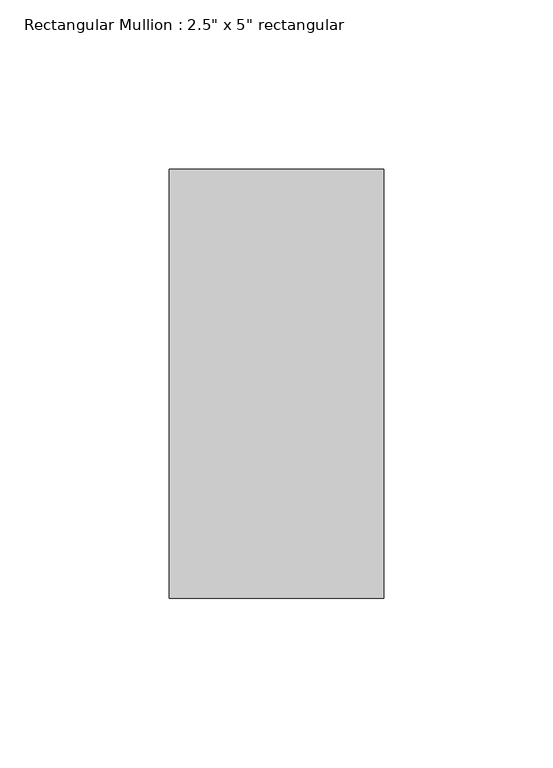
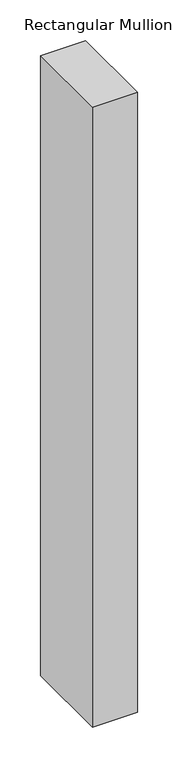
"""IFC4 building model written with IfcOpenShell, lengths in millimetres: member geometry."""

from ifc_helpers import new_model, si_unit, frame, origin, place, context, project, spatial, polyline, outline, extrude, source, transform, mapped, element, save


def member_e6e30476(model_context):
    return source(origin(), model_context, "Body", "SweptSolid", [
        extrude(outline(polyline([(0.0, 63.5), (0.0, -63.5), (-63.5, -63.5), (-63.5, 63.5), (0.0, 63.5)])), frame((0.0, 0.0, -927.3653615), z_axis=(0.0, 0.0, 1.0), x_axis=(1.0, 0.0, 0.0)), (0.0, 0.0, 1.0), 927.3653615),
    ])


if __name__ == "__main__":
    model = new_model("IFC4")
    model_context = context("Model", 3, world=origin())
    ifc_project = project(units=[si_unit("LENGTHUNIT", "METRE", prefix="MILLI")], contexts=[model_context])
    site = spatial("IfcSite", under=ifc_project)
    building = spatial("IfcBuilding", under=site)
    placement = place(None, origin())
    member_shape = member_e6e30476(model_context)
    element("IfcMember", 1, ObjectType="Rectangular Mullion : 2.5\" x 5\" rectangular", at=placement, inside=building, context=model_context, shape_type="MappedRepresentation", body=[
        mapped(member_shape, transform((0.0, 0.0, 0.0), x_axis=(1.0, 0.0, 0.0), y_axis=(0.0, 1.0, 0.0), z_axis=(0.0, 0.0, 1.0))),
    ])
    save(model, "model.ifc")

# Revit data of these elements
# Type "Rectangular Mullion : 2.5\" x 5\" rectangular"
#   built-in parameter 1007304 = 0.416667 (stored number, unit not read)
#   built-in parameter 1007301 = 0.104167 (stored number, unit not read)
#   built-in parameter 1007300 = 0.104167 (stored number, unit not read)
# Element 1 (IfcMember, "Rectangular Mullion : 2.5\" x 5\" rectangular")
#   Materials on its faces: "Aluminum"
# Materials
#   "Aluminum": class "Metal", colour RGB 247 247 247, transparency 0, Description = "Aluminum 6061", Cost = 0
